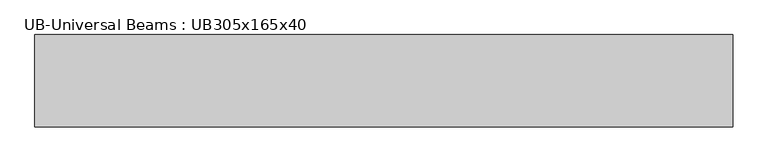
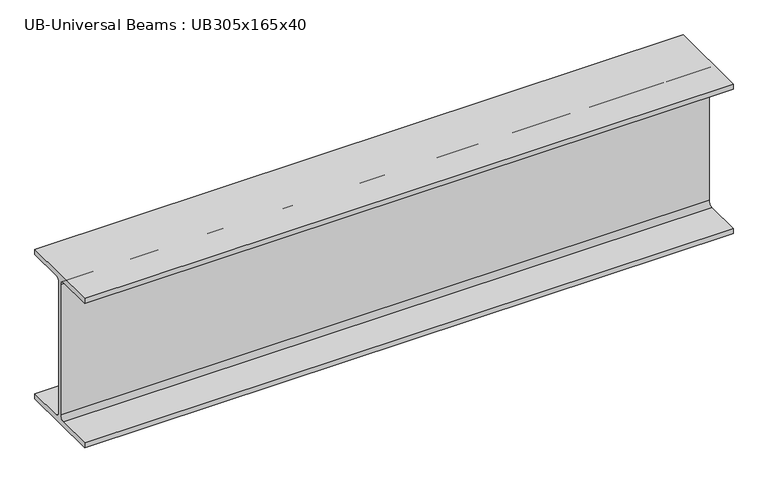
"""IFC4 building model written with IfcOpenShell, lengths in millimetres: beam geometry, UB-Universal Beams : UB305x165x40."""

from ifc_helpers import new_model, si_unit, point, frame, frame_2d, origin, place, context, project, spatial, polyline, circle_curve, trimmed, segment, composite_curve, outline, extrude, source, transform, mapped, element, save


def ub_universal_beams_ub305x165x40_7abb9ae2(model_context):
    return source(origin(), model_context, "Body", "SweptSolid", [
        extrude(outline(composite_curve([segment(polyline([(82.5, -141.5), (82.5, -151.7), (-82.5, -151.7), (-82.5, -141.5), (-11.9, -141.5)]), True, "CONTINUOUS"), segment(trimmed(circle_curve(frame_2d((-11.9, -132.6)), 8.9), [point((-11.9, -141.5))], [point((-3.0, -132.6))], True, "CARTESIAN"), True, "CONTINUOUS"), segment(polyline([(-3.0, -132.6), (-3.0, 132.6)]), True, "CONTINUOUS"), segment(trimmed(circle_curve(frame_2d((-11.9, 132.6)), 8.9), [point((-3.0, 132.6))], [point((-11.9, 141.5))], True, "CARTESIAN"), True, "CONTINUOUS"), segment(polyline([(-11.9, 141.5), (-82.5, 141.5), (-82.5, 151.7), (82.5, 151.7), (82.5, 141.5), (11.9, 141.5)]), True, "CONTINUOUS"), segment(trimmed(circle_curve(frame_2d((11.9, 132.6)), 8.9), [point((11.9, 141.5))], [point((3.0, 132.6))], True, "CARTESIAN"), True, "CONTINUOUS"), segment(polyline([(3.0, 132.6), (3.0, -132.6)]), True, "CONTINUOUS"), segment(trimmed(circle_curve(frame_2d((11.9, -132.6)), 8.9), [point((3.0, -132.6))], [point((11.9, -141.5))], True, "CARTESIAN"), True, "CONTINUOUS"), segment(polyline([(11.9, -141.5), (82.5, -141.5)]), True, "CONTINUOUS")], self_intersect=False)), frame((-635.6, 0.0, 0.0), z_axis=(1.0, 0.0, 0.0), x_axis=(0.0, 1.0, 0.0)), (0.0, 0.0, 1.0), 1245.4),
    ])


if __name__ == "__main__":
    model = new_model("IFC4")
    model_context = context("Model", 3, world=origin())
    ifc_project = project(units=[si_unit("LENGTHUNIT", "METRE", prefix="MILLI")], contexts=[model_context])
    site = spatial("IfcSite", under=ifc_project)
    building = spatial("IfcBuilding", under=site)
    placement = place(None, origin())
    ub_universal_beams_ub305x165x40_shape = ub_universal_beams_ub305x165x40_7abb9ae2(model_context)
    element("IfcBeam", 1, ObjectType="UB-Universal Beams : UB305x165x40", at=placement, inside=building, context=model_context, shape_type="MappedRepresentation", body=[
        mapped(ub_universal_beams_ub305x165x40_shape, transform((0.0, 0.0, 0.0), x_axis=(1.0, 0.0, 0.0), y_axis=(0.0, 1.0, 0.0), z_axis=(0.0, 0.0, 1.0))),
    ])
    save(model, "model.ifc")

# Revit data of these elements
# Type "UB-Universal Beams : UB305x165x40"
#   Section Name Key = "UB305X165X40"
#   Width = 16.5 cm
#   Web Thickness = 0.6 cm
#   Web Fillet = 0.89 cm
#   Warping Constant = 164000.0 cm⁶
#   Torsional Moment of Inertia = 14.70 cm⁴
#   Section Area = 51.3 cm²
#   Plastic Modulus weak axis = 142.0 cm³
#   Plastic Modulus strong axis = 623.0 cm³
#   Nominal Weight = 40.2999 kgf/m
#   Moment of Inertia weak axis = 764.00 cm⁴
#   Moment of Inertia strong axis = 8503.00 cm⁴
#   Height = 30.34 cm
#   Flange Thickness = 1.02 cm
#   Elastic Modulus weak axis = 92.6 cm³
#   Elastic Modulus strong axis = 560.0 cm³
#   Centroid Vertical = 15.17 cm
#   Centroid Horizontal = 8.25 cm
#   Bolt Spacing = 9.0 cm
#   Length [instance default] = 1500 mm
#   Structural Material [instance default] = Metal - Steel 43-275
#   Type Comments = ""
#   Assembly Code = ""
# Element 1 (IfcBeam, "UB-Universal Beams : UB305x165x40")
#   Materials on its faces: "Metal - Steel 43-275"
# Materials
#   "Metal - Steel 43-275": class "Metal", colour RGB 247 247 247, transparency 0, Cost = 0
